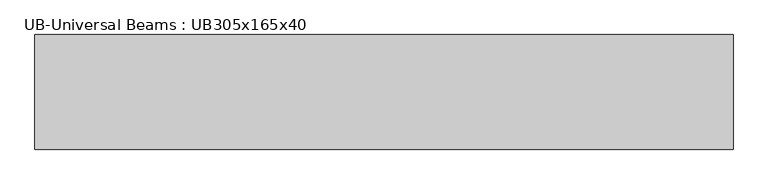
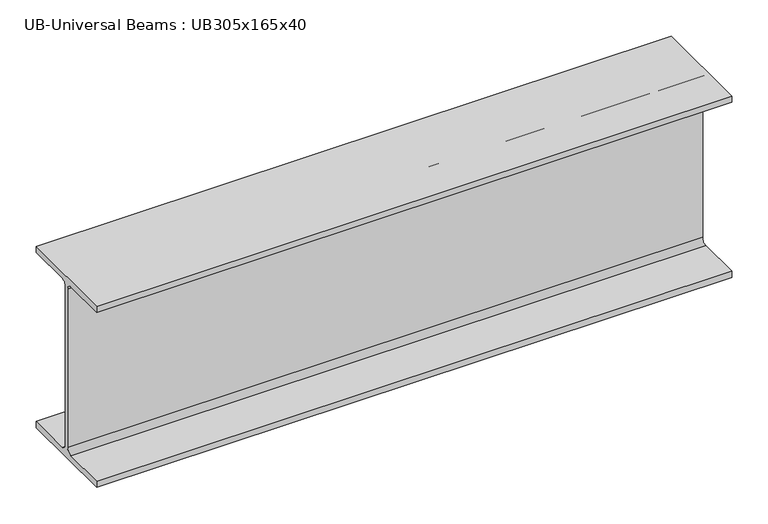
"""IFC4 building model written with IfcOpenShell, lengths in millimetres: beam geometry, UB-Universal Beams : UB305x165x40."""

from ifc_helpers import new_model, si_unit, point, frame, frame_2d, origin, place, context, project, spatial, polyline, circle_curve, trimmed, segment, composite_curve, outline, extrude, source, transform, mapped, element, save


def ub_universal_beams_ub305x165x40_9b118c67(model_context):
    return source(origin(), model_context, "Body", "SweptSolid", [
        extrude(outline(composite_curve([segment(polyline([(82.5, -141.5), (82.5, -151.7), (-82.5, -151.7), (-82.5, -141.5), (-11.9, -141.5)]), True, "CONTINUOUS"), segment(trimmed(circle_curve(frame_2d((-11.9, -132.6)), 8.9), [point((-11.9, -141.5))], [point((-3.0, -132.6))], True, "CARTESIAN"), True, "CONTINUOUS"), segment(polyline([(-3.0, -132.6), (-3.0, 132.6)]), True, "CONTINUOUS"), segment(trimmed(circle_curve(frame_2d((-11.9, 132.6)), 8.9), [point((-3.0, 132.6))], [point((-11.9, 141.5))], True, "CARTESIAN"), True, "CONTINUOUS"), segment(polyline([(-11.9, 141.5), (-82.5, 141.5), (-82.5, 151.7), (82.5, 151.7), (82.5, 141.5), (11.9, 141.5)]), True, "CONTINUOUS"), segment(trimmed(circle_curve(frame_2d((11.9, 132.6)), 8.9), [point((11.9, 141.5))], [point((3.0, 132.6))], True, "CARTESIAN"), True, "CONTINUOUS"), segment(polyline([(3.0, 132.6), (3.0, -132.6)]), True, "CONTINUOUS"), segment(trimmed(circle_curve(frame_2d((11.9, -132.6)), 8.9), [point((3.0, -132.6))], [point((11.9, -141.5))], True, "CARTESIAN"), True, "CONTINUOUS"), segment(polyline([(11.9, -141.5), (82.5, -141.5)]), True, "CONTINUOUS")], self_intersect=False)), frame((-332.1, 0.0, 0.0), z_axis=(1.0, 0.0, 0.0), x_axis=(0.0, 1.0, 0.0)), (0.0, 0.0, 1.0), 1004.9),
    ])


if __name__ == "__main__":
    model = new_model("IFC4")
    model_context = context("Model", 3, world=origin())
    ifc_project = project(units=[si_unit("LENGTHUNIT", "METRE", prefix="MILLI")], contexts=[model_context])
    site = spatial("IfcSite", under=ifc_project)
    building = spatial("IfcBuilding", under=site)
    placement = place(None, origin())
    ub_universal_beams_ub305x165x40_shape = ub_universal_beams_ub305x165x40_9b118c67(model_context)
    element("IfcBeam", 1, ObjectType="UB-Universal Beams : UB305x165x40", at=placement, inside=building, context=model_context, shape_type="MappedRepresentation", body=[
        mapped(ub_universal_beams_ub305x165x40_shape, transform((0.0, 0.0, 0.0), x_axis=(1.0, 0.0, 0.0), y_axis=(0.0, 1.0, 0.0), z_axis=(0.0, 0.0, 1.0))),
    ])
    save(model, "model.ifc")

# Revit data of these elements
# Type "UB-Universal Beams : UB305x165x40"
#   Section Name Key = "UB305X165X40"
#   Width = 16.5 cm
#   Web Thickness = 0.6 cm
#   Web Fillet = 0.89 cm
#   Warping Constant = 164000.0 cm⁶
#   Torsional Moment of Inertia = 14.70 cm⁴
#   Section Area = 51.3 cm²
#   Plastic Modulus weak axis = 142.0 cm³
#   Plastic Modulus strong axis = 623.0 cm³
#   Nominal Weight = 40.2999 kgf/m
#   Moment of Inertia weak axis = 764.00 cm⁴
#   Moment of Inertia strong axis = 8503.00 cm⁴
#   Height = 30.34 cm
#   Flange Thickness = 1.02 cm
#   Elastic Modulus weak axis = 92.6 cm³
#   Elastic Modulus strong axis = 560.0 cm³
#   Centroid Vertical = 15.17 cm
#   Centroid Horizontal = 8.25 cm
#   Bolt Spacing = 9.0 cm
#   Length [instance default] = 1500 mm
#   Structural Material [instance default] = Metal - Steel 43-275
#   Type Comments = ""
#   Assembly Code = ""
# Element 1 (IfcBeam, "UB-Universal Beams : UB305x165x40")
#   Materials on its faces: "Metal - Steel 43-275"
# Materials
#   "Metal - Steel 43-275": class "Metal", colour RGB 247 247 247, transparency 0, Cost = 0
